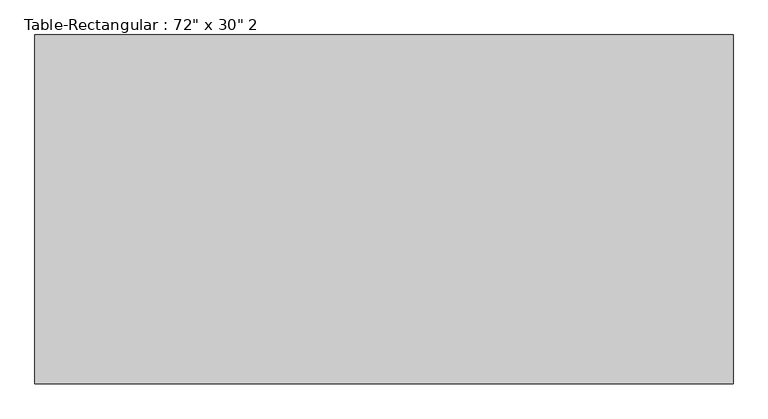
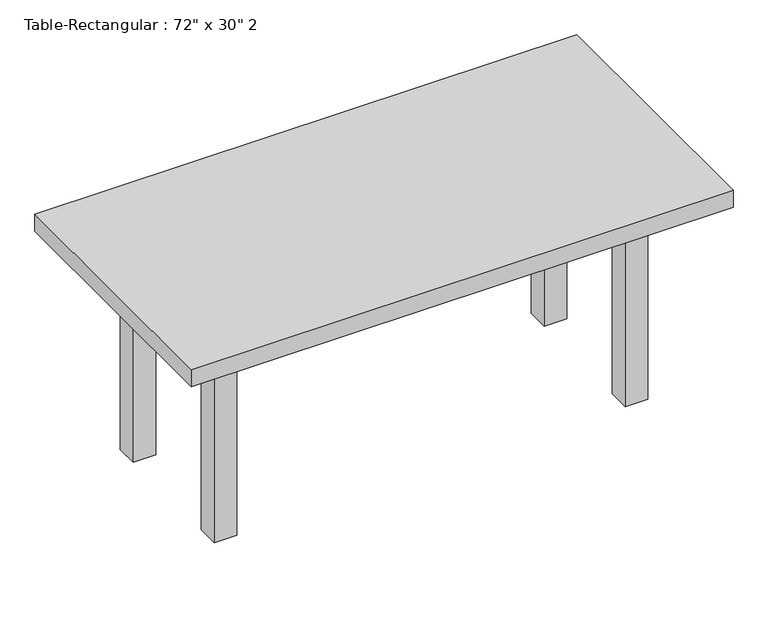
"""IFC4 building model written with IfcOpenShell, lengths in millimetres: furniture geometry."""

from ifc_helpers import new_model, si_unit, frame, origin, origin_with_axes, place, context, project, spatial, polyline, outline, extrude, source, transform, mapped, element, save


def furniture_2bbcfec9(model_context):
    return source(origin(), model_context, "Body", "SweptSolid", [
        extrude(outline(polyline([(546.1, 190.5), (546.1, 165.1), (-546.1, 165.1), (-546.1, 190.5), (546.1, 190.5)])), frame((0.0, 0.0, 508.0), z_axis=(0.0, 0.0, 1.0), x_axis=(1.0, 0.0, 0.0)), (0.0, 0.0, 1.0), 101.6),
        extrude(outline(polyline([(546.1, -190.5), (-546.1, -190.5), (-546.1, -165.1), (546.1, -165.1), (546.1, -190.5)])), frame((0.0, 0.0, 508.0), z_axis=(0.0, 0.0, 1.0), x_axis=(1.0, 0.0, 0.0)), (0.0, 0.0, 1.0), 101.6),
        extrude(outline(polyline([(-558.8, -165.1), (-584.2, -165.1), (-584.2, 165.1), (-558.8, 165.1), (-558.8, -165.1)])), frame((0.0, 0.0, 508.0), z_axis=(0.0, 0.0, 1.0), x_axis=(1.0, 0.0, 0.0)), (0.0, 0.0, 1.0), 101.6),
        extrude(outline(polyline([(558.8, -165.1), (558.8, 165.1), (584.2, 165.1), (584.2, -165.1), (558.8, -165.1)])), frame((0.0, 0.0, 508.0), z_axis=(0.0, 0.0, 1.0), x_axis=(1.0, 0.0, 0.0)), (0.0, 0.0, 1.0), 101.6),
        extrude(outline(polyline([(762.0, 381.0), (762.0, -381.0), (-762.0, -381.0), (-762.0, 381.0), (762.0, 381.0)])), frame((0.0, 0.0, 609.6), z_axis=(0.0, 0.0, 1.0), x_axis=(1.0, 0.0, 0.0)), (0.0, 0.0, 1.0), 50.8),
        extrude(outline(polyline([(-546.1, 228.6), (-546.1, 165.1), (-609.6, 165.1), (-609.6, 228.6), (-546.1, 228.6)])), origin_with_axes(), (0.0, 0.0, 1.0), 609.6),
        extrude(outline(polyline([(546.1, 228.6), (609.6, 228.6), (609.6, 165.1), (546.1, 165.1), (546.1, 228.6)])), origin_with_axes(), (0.0, 0.0, 1.0), 609.6),
        extrude(outline(polyline([(-546.1, -228.6), (-609.6, -228.6), (-609.6, -165.1), (-546.1, -165.1), (-546.1, -228.6)])), origin_with_axes(), (0.0, 0.0, 1.0), 609.6),
        extrude(outline(polyline([(546.1, -228.6), (546.1, -165.1), (609.6, -165.1), (609.6, -228.6), (546.1, -228.6)])), origin_with_axes(), (0.0, 0.0, 1.0), 609.6),
    ])


if __name__ == "__main__":
    model = new_model("IFC4")
    model_context = context("Model", 3, world=origin())
    ifc_project = project(units=[si_unit("LENGTHUNIT", "METRE", prefix="MILLI")], contexts=[model_context])
    site = spatial("IfcSite", under=ifc_project)
    building = spatial("IfcBuilding", under=site)
    placement = place(None, origin())
    furniture_shape = furniture_2bbcfec9(model_context)
    element("IfcFurniture", 1, ObjectType="Table-Rectangular : 72\" x 30\" 2", at=placement, inside=building, context=model_context, shape_type="MappedRepresentation", body=[
        mapped(furniture_shape, transform((0.0, 0.0, 0.0), x_axis=(1.0, 0.0, 0.0), y_axis=(0.0, 1.0, 0.0), z_axis=(0.0, 0.0, 1.0))),
    ])
    save(model, "model.ifc")

# Revit data of these elements
# Type "Table-Rectangular : 72\" x 30\" 2"
#   Assembly Code = "E2020200"
#   Height = 2' - 2"
#   Length = 5' - 0"
#   Width = 2' - 6"
#   Base Material = Birch
#   Top Material = Birch
#   Default Elevation = 0
# Element 1 (IfcFurniture, "Table-Rectangular : 72\" x 30\" 2")
#   Materials on its faces: "Birch"
# Materials
#   "Birch": class "Wood", colour RGB 210 159 95, transparency 0, Description = "Betula Alleghaniensis", Cost = 0
